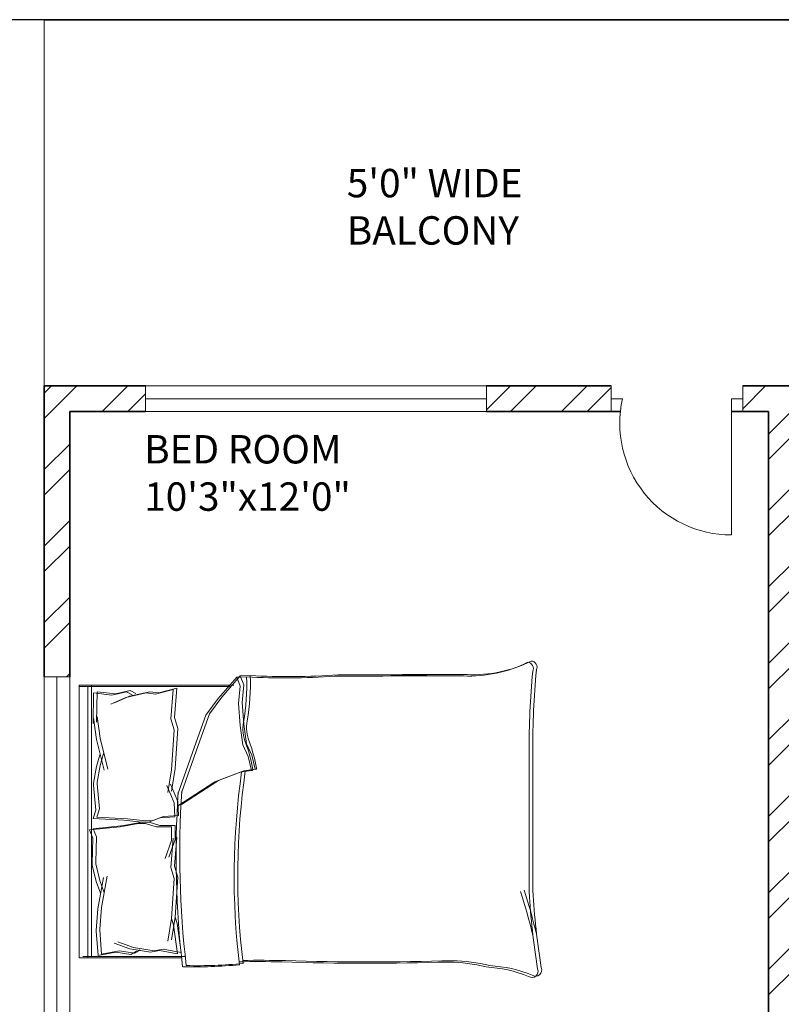
# Model space of a CAD drawing. Units: inches. Extents: x 2168 to 3056, y 1130 to 2629.
# Tile 23 of 42: x 2327 to 2462, y 2305 to 2478. Entities that reach past the tile are written whole.
import ezdxf

# ---------------------------------------------------------------- set-up
doc = ezdxf.new("R2010")
doc.units = ezdxf.units.IN
for name, color, linetype, lineweight in [('A-ANNO-DIMS', 2, 'Continuous', 18), ('A-AREA-IDEN', 7, 'Continuous', 18), ('A-DOOR', 21, 'Continuous', 18), ('A-FLOR-OTLN', 7, 'Continuous', 18), ('A-FURN', 8, 'Continuous', 13), ('A-GLAZ', 201, 'Continuous', 18), ('A-WALL', 7, 'Continuous', 35)]:
    doc.layers.add(name, color=color, linetype=linetype, lineweight=lineweight)
doc.layers.add('A-WALL-PATT', color=143, linetype='Continuous', lineweight=13, true_color=0x7aafdf)
doc.styles.get("Standard").update_dxf_attribs({"font": 'arial.ttf'})
doc.dimstyles.get("Standard").update_dxf_attribs({"dimtxt": 0.18, "dimasz": 0.18, "dimexe": 0.18, "dimexo": 0.0625, "dimgap": 0.09, "dimtad": 0, "dimtih": 1, "dimtoh": 1, "dimdec": 4, "dimzin": 0, "dimdsep": 46, "dimtxsty": 'Standard', "dimcen": 0.09, "dimadec": 0, "dimazin": 0, "dimtfac": 1, "dimtdec": 4, "dimtofl": 0, "dimtmove": 0, "dimatfit": 3, "dimfxl": 1, "dimtolj": 1, "dimtzin": 0, "dimarcsym": 0})

# ---------------------------------------------------------------- blocks, each defined once
blk = doc.blocks.new('BED-DOUBLE')
for p, q in [((27.75, 52.87), (24.5, 49.16)), ((27.75, 52.87), (24.5, 49.16)), ((28.39, 53.1), (25.14, 49.39)), ((28.39, 53.1), (25.14, 49.39)), ((29.49, 52.95), (27.75, 52.87, 3.87)), ((29.49, 52.95), (27.75, 52.87, 3.87)), ((28.37, 51.33), (27.75, 52.87)), ((28.37, 51.33), (27.75, 52.87)), ((30.13, 53.18), (28.39, 53.1, 3.87)), ((30.13, 53.18), (28.39, 53.1, 3.87)), ((29, 51.56), (28.39, 53.1)), ((29, 51.56), (28.39, 53.1)), ((0, 51.49), (0.64, 51.49)), ((0, 3.48), (0, 51.49)), ((0, 51.27), (26.61, 51.27)), ((0, 51.27), (26.61, 51.27)), ((0.64, 51.49), (27.25, 51.49)), ((0.64, 51.49), (27.25, 51.49)), ((1.53, 3.48), (1.53, 51.27)), ((1.53, 3.48), (1.53, 51.27)), ((2.17, 3.7), (2.17, 51.49)), ((2.17, 3.7), (2.17, 51.49)), ((3.2, 50.34), (3.1, 44.94)), ((3.2, 50.34), (3.1, 44.94)), ((3.2, 50.34), (6.41, 49.96)), ((3.2, 50.34), (6.41, 49.96)), ((5.77, 49.73), (8.34, 50.33)), ((5.77, 49.73), (8.34, 50.33)), ((6.41, 49.96), (8.98, 50.56)), ((6.41, 49.96), (8.98, 50.56)), ((8.34, 50.33), (9.38, 49.81)), ((8.34, 50.33), (9.38, 49.81)), ((12.47, 50.34), (8.9, 49.54)), ((12.47, 50.34), (8.9, 49.54)), ((8.98, 50.56), (10.02, 50.04)), ((8.98, 50.56), (10.02, 50.04)), ((14.07, 50.15), (12.47, 50.34)), ((14.07, 50.15), (12.47, 50.34)), ((16.57, 50.7), (13.43, 49.92)), ((16.57, 50.7), (13.43, 49.92)), ((17.21, 50.93), (14.07, 50.15)), ((17.21, 50.93), (14.07, 50.15)), ((16.17, 45.57), (16.57, 50.7)), ((16.17, 45.57), (16.57, 50.7)), ((16.81, 45.8), (17.21, 50.93)), ((16.81, 45.79), (17.21, 50.93)), ((28.06, 48.23), (28.37, 51.33)), ((28.06, 48.23), (28.37, 51.33)), ((28.7, 48.46), (29, 51.56)), ((28.7, 48.46), (29, 51.56)), ((2.56, 50.11), (2.46, 44.71)), ((2.56, 50.11), (2.46, 44.71)), ((2.56, 50.11), (5.77, 49.73)), ((2.56, 50.11), (5.77, 49.73)), ((8.26, 49.31), (5.58, 48.13)), ((8.26, 49.31), (5.58, 48.13)), ((8.9, 49.54), (6.22, 48.36)), ((8.9, 49.54), (6.22, 48.36)), ((11.83, 50.11), (8.26, 49.31)), ((11.83, 50.11), (8.26, 49.31)), ((13.43, 49.92), (11.83, 50.11)), ((13.43, 49.92), (11.83, 50.11)), ((24.5, 49.16), (22.33, 46.22)), ((24.5, 49.16), (22.33, 46.22)), ((25.14, 49.39), (22.97, 46.45)), ((25.14, 49.39), (22.97, 46.45)), ((28.37, 44.36), (28.06, 48.23)), ((28.37, 44.36), (28.06, 48.23)), ((29, 44.59), (28.7, 48.46)), ((29, 44.59), (28.7, 48.46)), ((2.46, 44.71), (2.54, 45.71)), ((2.46, 44.71), (2.54, 45.71)), ((2.54, 45.71), (3.07, 41.91)), ((2.54, 45.71), (3.07, 41.91)), ((3.1, 44.94), (3.18, 45.94)), ((3.1, 44.94), (3.18, 45.94)), ((3.18, 45.94), (3.71, 42.14)), ((3.18, 45.94), (3.71, 42.14)), ((16.73, 43.61), (16.17, 45.57)), ((16.73, 43.61), (16.17, 45.57)), ((17.37, 43.83), (16.81, 45.8)), ((17.37, 43.83), (16.81, 45.79)), ((22.33, 46.22), (20.32, 40.64)), ((22.33, 46.22), (20.32, 40.64)), ((22.97, 46.45), (20.96, 40.87)), ((22.97, 46.45), (20.96, 40.87)), ((16.3, 36.6), (16.73, 43.61)), ((16.3, 36.6), (16.73, 43.61)), ((16.93, 36.82), (17.37, 43.83)), ((16.93, 36.82), (17.37, 43.83)), ((28.83, 40.95), (28.37, 44.36)), ((28.83, 40.95), (28.37, 44.36)), ((29.47, 41.18), (29, 44.59)), ((29.47, 41.18), (29, 44.59)), ((3.07, 41.91), (4.42, 36.5)), ((3.07, 41.91), (4.42, 36.49)), ((3.71, 42.14), (5.06, 36.72)), ((3.71, 42.14), (5.06, 36.72)), ((20.32, 40.64), (17.38, 32.31)), ((20.32, 40.64), (17.38, 32.31)), ((20.96, 40.87), (18.02, 32.53)), ((20.96, 40.87), (18.02, 32.53)), ((29.76, 38.94), (28.83, 40.95)), ((29.76, 38.94), (28.83, 40.95)), ((30.4, 39.17), (29.47, 41.18)), ((30.4, 39.17), (29.47, 41.18)), ((79.88, 15.29), (79.88, 39.91)), ((79.88, 15.29), (79.88, 39.91)), ((3.67, 39.2), (3.08, 37.14)), ((3.67, 39.2), (3.08, 37.14)), ((4.31, 39.43), (3.72, 37.36)), ((4.31, 39.43), (3.72, 37.36)), ((30.38, 36.46), (29.76, 38.94)), ((30.38, 36.46), (29.76, 38.94)), ((31.02, 36.69), (30.4, 39.17)), ((31.02, 36.69), (30.4, 39.17)), ((79.25, 15.06), (79.25, 39.68)), ((79.25, 15.06), (79.25, 39.68)), ((3.08, 37.14), (2.54, 34.2)), ((3.08, 37.14), (2.54, 34.2)), ((3.72, 37.36), (3.18, 34.43)), ((3.72, 37.36), (3.18, 34.43)), ((15.63, 32.56), (16.3, 36.6)), ((15.63, 32.56), (16.3, 36.6)), ((16.27, 32.79), (16.93, 36.82)), ((16.27, 32.79), (16.93, 36.82)), ((28.37, 36.15), (30.38, 36.46)), ((28.37, 36.15), (30.38, 36.46)), ((29, 36.38), (31.02, 36.69)), ((29, 36.38), (31.02, 36.69)), ((23.88, 34.45), (28.37, 36.15)), ((23.88, 34.45), (28.37, 36.15)), ((24.52, 34.68), (29, 36.38)), ((24.52, 34.68), (29, 36.38)), ((2.54, 34.2), (2.56, 33.88)), ((2.54, 34.2), (2.56, 33.88)), ((2.56, 33.88), (2.98, 29.46)), ((2.56, 33.88), (2.98, 29.46)), ((3.18, 34.43), (3.2, 34.11)), ((3.18, 34.43), (3.2, 34.11)), ((3.2, 34.11), (3.62, 29.68)), ((3.2, 34.11), (3.62, 29.68)), ((16.74, 30.75), (15.45, 33.82)), ((16.74, 30.75), (15.45, 33.82)), ((17.38, 30.98), (16.09, 34.05)), ((17.38, 30.98), (16.09, 34.05)), ((17.38, 30.26), (23.88, 34.45)), ((17.38, 30.26), (23.88, 34.45)), ((18.02, 30.49), (24.52, 34.68)), ((18.02, 30.49), (24.52, 34.68)), ((3.62, 29.68), (3.13, 28.21)), ((3.62, 29.68), (3.13, 28.21)), ((16.89, 28.3), (16.74, 30.75)), ((16.89, 28.3), (16.74, 30.75)), ((17.53, 28.53), (17.38, 30.98)), ((17.53, 28.53), (17.38, 30.98)), ((2.98, 29.46), (2.49, 27.98)), ((2.98, 29.46), (2.49, 27.98)), ((2.49, 27.98), (7.87, 27.73)), ((2.49, 27.98), (7.87, 27.73)), ((3.13, 28.21), (8.51, 27.96)), ((3.13, 28.21), (8.51, 27.96)), ((8.51, 27.96), (11.72, 27.58)), ((8.51, 27.96), (11.72, 27.58)), ((12.38, 27.44), (14.22, 28.13)), ((12.38, 27.44), (14.22, 28.13)), ((13.02, 27.66), (14.86, 28.36)), ((13.02, 27.66), (14.86, 28.36)), ((14.22, 28.13), (16.89, 28.3)), ((14.22, 28.13), (16.89, 28.3)), ((14.86, 28.36), (17.53, 28.53)), ((14.86, 28.36), (17.53, 28.53)), ((1.87, 25.98), (7.22, 26.56)), ((1.87, 25.98), (7.22, 26.56)), ((2.51, 26.21), (7.86, 26.79)), ((2.51, 26.21), (7.86, 26.79)), ((3.09, 24.77), (2.51, 26.21)), ((3.09, 24.77), (2.51, 26.21)), ((7.22, 26.56), (10.4, 27.14)), ((7.22, 26.56), (10.4, 27.14)), ((7.86, 26.79), (11.04, 27.37)), ((7.86, 26.79), (11.04, 27.37)), ((7.87, 27.73), (11.08, 27.36)), ((7.87, 27.73), (11.08, 27.35)), ((10.4, 27.14), (11.7, 27.14)), ((10.4, 27.14), (11.7, 27.14)), ((11.04, 27.37), (12.34, 27.37)), ((11.04, 27.37), (12.34, 27.37)), ((11.08, 27.36), (12.38, 27.44)), ((11.08, 27.35), (12.38, 27.44)), ((11.7, 27.14), (13.58, 26.56)), ((11.7, 27.14), (13.58, 26.56)), ((11.72, 27.58), (13.02, 27.66)), ((11.72, 27.58), (13.02, 27.66)), ((12.34, 27.37), (14.22, 26.79)), ((12.34, 27.37), (14.22, 26.79)), ((13.58, 26.56), (16.26, 26.56)), ((13.58, 26.56), (16.26, 26.56)), ((14.22, 26.79), (16.9, 26.79)), ((14.22, 26.79), (16.9, 26.79)), ((16.26, 26.56), (16.26, 24.1)), ((16.26, 26.56), (16.26, 24.1)), ((16.9, 26.79), (16.9, 24.33)), ((16.9, 26.79), (16.9, 24.33)), ((2.45, 24.54), (1.87, 25.98)), ((2.45, 24.54), (1.87, 25.98)), ((2.3, 20.09), (2.45, 24.54)), ((2.3, 20.09), (2.45, 24.54)), ((2.94, 20.32), (3.09, 24.77)), ((2.94, 20.32), (3.09, 24.77)), ((16.9, 24.33), (15.81, 21.19)), ((16.9, 24.33), (15.81, 21.19)), ((16.17, 19.38), (16.57, 24.52)), ((16.17, 19.38), (16.57, 24.52)), ((16.81, 19.61), (17.21, 24.74)), ((16.81, 19.61), (17.21, 24.74)), ((16.26, 24.1), (15.17, 20.96)), ((16.26, 24.1), (15.17, 20.96)), ((2.3, 19.77), (2.3, 20.09)), ((2.3, 19.77), (2.3, 20.09)), ((3.03, 16.88), (2.3, 19.77)), ((3.03, 16.88), (2.3, 19.77)), ((2.94, 20), (2.94, 20.32)), ((2.94, 20), (2.94, 20.32)), ((3.67, 17.11), (2.94, 20)), ((3.67, 17.11), (2.94, 20)), ((16.73, 17.42), (16.17, 19.38)), ((16.73, 17.42), (16.17, 19.38)), ((17.37, 17.65), (16.81, 19.61)), ((17.37, 17.65), (16.81, 19.61)), ((3.32, 12.11), (4.33, 17.6)), ((3.32, 12.11), (4.33, 17.6)), ((3.96, 12.34), (4.97, 17.83)), ((3.96, 12.34), (4.97, 17.83)), ((16.3, 10.41), (16.73, 17.42)), ((16.3, 10.41), (16.73, 17.42)), ((16.93, 10.64), (17.37, 17.65)), ((16.93, 10.64), (17.37, 17.65)), ((3.75, 14.86), (3.03, 16.88)), ((3.75, 14.85), (3.03, 16.88)), ((4.39, 15.08), (3.67, 17.11)), ((4.39, 15.08), (3.67, 17.11)), ((3.67, 8.51), (3.96, 12.34)), ((3.67, 8.51), (3.96, 12.34)), ((3.03, 8.29), (3.32, 12.11)), ((3.03, 8.28), (3.32, 12.11)), ((15.63, 6.38), (16.3, 10.41)), ((15.63, 6.38), (16.3, 10.41)), ((16.27, 6.61), (16.93, 10.64)), ((16.27, 6.61), (16.93, 10.64)), ((16.3, 10.41), (16.62, 9.28)), ((16.3, 10.41), (16.62, 9.28)), ((16.93, 10.64), (17.26, 9.51)), ((16.93, 10.64), (17.26, 9.51)), ((16.62, 9.28), (17.34, 4.18)), ((16.62, 9.28), (17.34, 4.18)), ((17.26, 9.51), (17.98, 4.41)), ((17.26, 9.51), (17.98, 4.41)), ((3.01, 8.18), (3.03, 8.29)), ((3.01, 8.18), (3.03, 8.28)), ((3.34, 3.9), (3.01, 8.18)), ((3.34, 3.9), (3.01, 8.18)), ((3.65, 8.41), (3.67, 8.51)), ((3.65, 8.41), (3.67, 8.51)), ((3.98, 4.13), (3.65, 8.41)), ((3.98, 4.13), (3.65, 8.41)), ((8.96, 5.05), (6.21, 6.06)), ((8.96, 5.05), (6.21, 6.06)), ((9.59, 5.28), (6.85, 6.29)), ((9.59, 5.28), (6.85, 6.29)), ((13.21, 4.7), (9.59, 5.28)), ((13.21, 4.7), (9.59, 5.28)), ((18.11, 3.48), (0, 3.48)), ((18.11, 3.48), (0, 3.48)), ((18.75, 3.7), (0.64, 3.7)), ((18.75, 3.7), (0.64, 3.7)), ((3.32, 3.89), (6.5, 4.47)), ((3.32, 3.89), (6.5, 4.47)), ((3.96, 4.12), (7.14, 4.7)), ((3.96, 4.12), (7.14, 4.7)), ((6.5, 4.47), (9.1, 4.04)), ((6.5, 4.47), (9.1, 4.04)), ((7.14, 4.7), (9.74, 4.27)), ((7.14, 4.7), (9.74, 4.27)), ((12.57, 4.47), (8.96, 5.05)), ((12.57, 4.47), (8.96, 5.05)), ((9.1, 4.04), (10.11, 4.62)), ((9.1, 4.04), (10.11, 4.62)), ((9.74, 4.27), (10.75, 4.85)), ((9.74, 4.27), (10.75, 4.85)), ((14.16, 4.76), (12.57, 4.47)), ((14.16, 4.76), (12.57, 4.47)), ((14.8, 4.99), (13.21, 4.7)), ((14.8, 4.99), (13.21, 4.7)), ((17.34, 4.18), (14.16, 4.76)), ((17.34, 4.18), (14.16, 4.76)), ((17.98, 4.41), (14.8, 4.99)), ((17.98, 4.41), (14.8, 4.99))]:
    blk.add_line(p, q)
for centre, radius, start, end in [((68.67, 76.16), 23.07, 267.4714, 296.4681), ((68.67, 76.16), 23.07, 267.4714, 296.4681), ((69.31, 76.39), 23.07, 267.4714, 296.4681), ((69.31, 76.39), 23.07, 267.4714, 296.4681), ((78.87, 54.41), 1.1, 332.6588, 86.02), ((78.87, 54.41), 1.1, 332.6588, 86.02), ((79.51, 54.64), 1.1, 332.6588, 86.02), ((79.51, 54.64), 1.1, 332.6588, 86.02), ((212.28, 41.15), 133.04, 174.4998, 180.6351), ((212.28, 41.15), 133.04, 174.4998, 180.6351), ((212.92, 41.38), 133.04, 174.4998, 180.6351), ((212.92, 41.38), 133.04, 174.4998, 180.6351), ((-6.66, 51.33), 36.18, 349.8763, 2.5657), ((-6.66, 51.33), 36.18, 349.8763, 2.5657), ((36.32, 182.27), 129.5, 266.9791, 273.8365), ((36.32, 182.27), 129.5, 266.9791, 273.8365), ((-6.02, 51.56), 36.18, 349.8763, 2.5657), ((-6.02, 51.56), 36.18, 349.8763, 2.5657), ((36.95, 182.49), 129.5, 266.9791, 273.8365), ((36.95, 182.49), 129.5, 266.9791, 273.8365), ((67.82, -4508.74), 4561.86, 90.00217, 90.28689), ((67.82, -4508.74), 4561.86, 90.00217, 90.28689), ((68.46, -4508.51), 4561.86, 90.00217, 90.28689), ((68.46, -4508.52), 4561.86, 90.00217, 90.28689), ((35.71, 43.97), 6.22, 168.6608, 203.7384), ((35.71, 43.97), 6.22, 168.6608, 203.7384), ((35.07, 43.74), 6.22, 168.6608, 203.7384), ((35.07, 43.74), 6.22, 168.6608, 203.7384), ((1.48, 31.15), 29.65, 10.6617, 19.8806), ((1.48, 31.15), 29.65, 10.6617, 19.8806), ((2.12, 31.38), 29.65, 10.6617, 19.8806), ((2.12, 31.38), 29.65, 10.6617, 19.8806), ((156.96, 17.98), 129.02, 171.7845, 186.9006), ((156.96, 17.98), 129.02, 171.7845, 186.9006), ((30.44, 36.64), 0.185, 250.2464, 1.1377), ((30.44, 36.64), 0.185, 250.2464, 1.1377), ((31.08, 36.86), 0.185, 250.2464, 1.1377), ((31.08, 36.86), 0.185, 250.2464, 1.1377), ((156.32, 17.76), 129.02, 171.7845, 186.9006), ((156.32, 17.76), 129.02, 171.7845, 186.9006), ((182.05, 21.36), 164.97, 176.0865, 186.7821), ((182.05, 21.36), 164.97, 176.0865, 186.7821), ((182.69, 21.59), 164.97, 176.0865, 186.7821), ((182.69, 21.59), 164.97, 176.0865, 186.7821), ((-23.71, -17.22), 106.46, 13.3832, 17.7053), ((-23.71, -17.22), 106.46, 13.3832, 17.7053), ((-23.07, -16.99), 106.46, 13.3832, 17.7053), ((-23.07, -16.99), 106.46, 13.3832, 17.7053), ((200.84, 21.43), 121.76, 182.9958, 189.4091), ((200.84, 21.43), 121.76, 182.9958, 189.4091), ((201.48, 21.66), 121.76, 182.9958, 189.4091), ((201.48, 21.66), 121.76, 182.9958, 189.4091), ((20.1, 85.16), 83.31, 268.7218, 275.604), ((20.1, 85.16), 83.31, 268.7218, 275.604), ((20.74, 85.39), 83.31, 268.7218, 275.604), ((20.74, 85.39), 83.31, 268.7218, 275.604), ((31.17, -167.31), 170.11, 88.4762, 91.0082), ((31.17, -167.31), 170.11, 88.4762, 91.0082), ((31.81, -167.08), 170.11, 88.4762, 91.0082), ((31.81, -167.08), 170.11, 88.4762, 91.0082), ((50.61, 484.82), 482.31, 268.2277, 271.7185), ((50.61, 484.82), 482.31, 268.2277, 271.7185), ((51.25, 485.05), 482.31, 268.2277, 271.7185), ((51.25, 485.05), 482.31, 268.2277, 271.7185), ((64.52, -26.9), 29.63, 76.0648, 88.9113), ((64.52, -26.9), 29.63, 76.0648, 88.9113), ((65.15, -26.67), 29.63, 76.0648, 88.9113), ((65.15, -26.67), 29.63, 76.0648, 88.9113), ((70.28, -21.66), 23.56, 67.9751, 86.652), ((70.28, -21.66), 23.56, 67.9751, 86.652), ((70.92, -21.43), 23.56, 67.9751, 86.652), ((70.92, -21.43), 23.56, 67.9751, 86.652), ((80.36, 1.32), 1.09, 236.1736, 23.4781), ((80.36, 1.32), 1.09, 236.1736, 23.4781), ((79.72, 1.09), 1.09, 236.1736, 23.4781), ((79.72, 1.09), 1.09, 236.1736, 23.4781)]:
    blk.add_arc(centre, radius, start, end)
blk = doc.blocks.new('WIN-60-OPPOSED-JAMBS')
for p, q in [((2.25, 60), (0, 60)), ((0, 60), (4.5, 60)), ((0, 60), (0, 0)), ((2.25, 0), (2.25, 60)), ((4.5, 60), (4.5, 0)), ((0, 0), (4.5, 0)), ((4.5, 0), (2.25, 0))]:
    blk.add_line(p, q)
blk = doc.blocks.new('*D41')
at = {"layer": 'A-ANNO-DIMS', "color": 0, "lineweight": -2, "transparency": 16777216}
for p, q in [((2331.73, 2478.39), (2273.32, 2478.39)), ((2273.5, 2478.21), (2273.5, 1928.07)), ((2273.5, 1377.57), (2273.5, 1927.71)), ((2331.73, 1377.39), (2273.32, 1377.39))]:
    blk.add_line(p, q, dxfattribs=at)
at = {"layer": 'A-ANNO-DIMS', "color": 0, "transparency": 16777216}
for points in [[(2273.47, 2478.21), (2273.53, 2478.21), (2273.5, 2478.39)], [(2273.47, 1377.57), (2273.53, 1377.57), (2273.5, 1377.39)]]:
    blk.add_solid(points, dxfattribs=at)
at = {"layer": 'Defpoints', "color": 0, "transparency": 16777216}
for p in [(2273.5, 2478.39), (2331.8, 2478.39), (2331.8, 1377.39)]:
    blk.add_point(p, dxfattribs=at)
at = {"layer": 'A-ANNO-DIMS', "color": 0, "transparency": 16777216, "insert": (2273.5, 1927.89), "char_height": 0.18, "attachment_point": 5}
blk.add_mtext('\\A1;1101', dxfattribs=at)

msp = doc.modelspace()

# ---------------------------------------------------------------- hatches: boundary and pattern name
at = {"layer": 'A-WALL-PATT'}
h = msp.add_hatch(dxfattribs=at)
h.set_pattern_fill('ANSI32', color=256)
h.paths.add_polyline_path([(2463.8, 2409.39), (2467.39, 2409.39), (2467.39, 2413.89), (2454.77, 2413.89), (2454.77, 2411.64), (2454.77, 2409.39), (2459.3, 2409.39), (2459.3, 2265.39), (2455.64, 2265.39), (2455.64, 2260.89), (2467.35, 2260.89), (2467.35, 2263.14), (2467.35, 2265.39), (2463.8, 2265.39)])
h.paths.add_polyline_path([(2431.6, 2413.89), (2409.65, 2413.89), (2409.65, 2409.39), (2431.6, 2409.39), (2431.6, 2411.64)])
h.paths.add_polyline_path([(2349.65, 2413.89), (2331.8, 2413.89), (2331.8, 2362.67), (2336.3, 2362.67), (2336.3, 2409.39), (2349.65, 2409.39), (2349.65, 2411.64)])
h.paths.add_polyline_path([(2634.15, 2411.64), (2634.15, 2413.89), (2562.29, 2413.89), (2562.29, 2409.39), (2595.8, 2409.39), (2595.8, 2280.31), (2595.83, 2280.31), (2595.83, 2265.39), (2499.91, 2265.39), (2499.91, 2260.89), (2550.8, 2260.89), (2550.8, 2117.31), (2555.3, 2117.31), (2555.3, 2168.08), (2571.93, 2168.08), (2571.93, 2176.89), (2559.8, 2176.89), (2559.8, 2256.39), (2640.8, 2256.39), (2640.8, 2176.89), (2626.43, 2176.89), (2626.43, 2168.08), (2645.3, 2168.08), (2645.3, 2116.64), (2649.8, 2116.64), (2649.8, 2260.89), (2691.25, 2260.89), (2691.25, 2263.14), (2691.25, 2265.39), (2670.65, 2265.39), (2670.65, 2265.36), (2600.3, 2265.36), (2600.3, 2280.26), (2600.3, 2409.39), (2634.15, 2409.39)])
h.paths.add_polyline_path([(2600.3, 2473.89), (2612.84, 2473.89), (2612.84, 2478.39), (2572.64, 2478.39), (2572.64, 2473.89), (2595.8, 2473.89), (2595.8, 2413.89), (2600.3, 2413.89)])
h.paths.add_polyline_path([(2535.8, 2473.89), (2548.64, 2473.89), (2548.64, 2478.39), (2531.4, 2478.39), (2531.4, 2413.89), (2521.6, 2413.89), (2521.6, 2409.39), (2539.24, 2409.39), (2539.24, 2411.64), (2539.24, 2413.89), (2535.8, 2413.89)])
h.paths.add_polyline_path([(2664.8, 2478.39), (2636.84, 2478.39), (2636.84, 2473.89), (2660.3, 2473.89), (2660.3, 2413.89), (2656.17, 2413.89), (2656.17, 2409.39), (2671.68, 2409.39), (2671.68, 2411.64), (2671.68, 2413.89), (2664.8, 2413.89)])
h.paths.add_polyline_path([(2705.94, 2413.89), (2695.68, 2413.89), (2695.68, 2409.39), (2705.94, 2409.39)])
h.paths.add_polyline_path([(2741.35, 2413.89), (2728.73, 2413.89), (2728.73, 2411.64), (2728.73, 2409.39), (2732.3, 2409.39), (2732.3, 2265.39), (2725.73, 2265.39), (2725.73, 2260.89), (2740.92, 2260.89), (2740.92, 2263.14), (2740.92, 2265.39), (2736.8, 2265.39), (2736.8, 2409.39), (2741.35, 2409.39)])
h.paths.add_polyline_path([(2785.65, 2413.89), (2764.55, 2413.89), (2764.49, 2409.39), (2785.65, 2409.39), (2785.65, 2411.64)])
h.paths.add_polyline_path([(2864.3, 2413.89), (2845.65, 2413.89), (2845.65, 2409.39), (2859.8, 2409.39), (2859.8, 2368.43), (2864.3, 2368.43)])
h.paths.add_polyline_path([(2864.3, 2308.43), (2862.05, 2308.43), (2859.8, 2308.43), (2859.8, 2265.39), (2774.48, 2265.39), (2774.48, 2263.14), (2774.48, 2260.89), (2781.8, 2260.89), (2781.8, 2226.65), (2786.3, 2226.65), (2786.3, 2260.89), (2859.8, 2260.89), (2859.8, 2241.35), (2864.3, 2241.35)])
h.paths.add_polyline_path([(2864.3, 2217.35), (2862.05, 2217.35), (2859.8, 2217.35), (2859.8, 2200.89), (2786.3, 2200.89), (2786.3, 2205.93), (2784.05, 2205.93), (2781.8, 2205.93), (2781.8, 2150.97), (2786.3, 2150.97), (2786.3, 2161.89), (2859.8, 2161.89), (2859.8, 2144.42), (2864.3, 2144.42)])
h.paths.add_polyline_path([(2859.8, 2196.39), (2859.8, 2166.39), (2786.3, 2166.39), (2786.3, 2196.39)], flags=16)
h.paths.add_polyline_path([(2864.3, 2108.42), (2862.05, 2108.42), (2859.8, 2108.42), (2859.8, 2080.89), (2786.3, 2080.89), (2786.3, 2111.99), (2781.8, 2111.99), (2781.8, 2080.89), (2649.8, 2080.89), (2649.8, 2086.04), (2647.55, 2086.04), (2645.3, 2086.04), (2645.3, 2071.74), (2649.8, 2071.74), (2649.8, 2076.39), (2781.8, 2076.39), (2781.8, 2041.79), (2786.3, 2041.79), (2786.3, 2076.39), (2859.8, 2076.39), (2859.8, 2058.58), (2864.3, 2058.58)])
h.paths.add_polyline_path([(2864.3, 2022.58), (2859.8, 2022.58), (2859.8, 1992.39), (2786.3, 1992.39), (2786.3, 1999.57), (2781.8, 1999.57), (2781.8, 1848.09), (2784.05, 1848.09), (2786.3, 1848.09), (2786.3, 1851.39), (2859.8, 1851.39), (2859.8, 1838.26), (2864.3, 1838.26)], flags=17)
h.paths.add_polyline_path([(2859.8, 1987.89), (2859.8, 1855.89), (2786.3, 1855.89), (2786.3, 1987.89)], flags=16)
h.paths.add_polyline_path([(2823.05, 1987.89), (2841.42, 1921.89), (2823.05, 1855.89)], flags=0)
h.paths.add_polyline_path([(2864.3, 1814.26), (2859.8, 1814.26), (2859.8, 1791.39), (2786.3, 1791.39), (2786.3, 1825.66), (2784.05, 1825.66), (2781.8, 1825.66), (2781.8, 1791.39), (2720.15, 1791.39), (2720.15, 1791.27), (2649.8, 1791.27), (2649.8, 1806.16), (2649.8, 2038.98), (2647.55, 2038.98), (2645.3, 2038.98), (2645.3, 1783.93), (2649.8, 1783.93), (2649.8, 1786.89), (2781.8, 1786.89), (2781.8, 1746.79), (2786.3, 1746.79), (2786.3, 1786.89), (2859.8, 1786.89), (2859.8, 1770.08), (2864.3, 1770.08)])
h.paths.add_polyline_path([(2864.3, 1734.08), (2862.05, 1734.08), (2859.8, 1734.08), (2859.8, 1705.89), (2786.3, 1705.89), (2786.3, 1714.17), (2781.8, 1714.17), (2781.8, 1660.53), (2786.3, 1660.53), (2786.3, 1666.89), (2859.8, 1666.89), (2859.8, 1648.34), (2864.3, 1648.34)])
h.paths.add_polyline_path([(2786.3, 1701.39), (2859.8, 1701.39), (2859.8, 1671.39), (2786.3, 1671.39)], flags=16)
h.paths.add_polyline_path([(2649.8, 1756.58), (2647.55, 1756.58), (2645.3, 1756.58), (2645.3, 1606.89), (2555.3, 1606.89), (2555.3, 1749.51), (2553.05, 1749.51), (2550.8, 1749.51), (2550.8, 1606.89), (2503.01, 1606.89), (2503.01, 1604.64), (2503.01, 1602.39), (2595.8, 1602.39), (2595.85, 1602.39), (2595.85, 1587.5), (2595.8, 1458.39), (2561.5, 1458.39), (2561.5, 1456.14), (2561.5, 1453.89), (2595.8, 1453.89), (2595.8, 1381.89), (2573.44, 1381.89), (2573.44, 1377.39), (2613.01, 1377.39), (2613.01, 1379.64), (2613.01, 1381.89), (2600.3, 1381.89), (2600.3, 1453.89), (2634.33, 1453.89), (2634.33, 1458.39), (2600.3, 1458.39), (2600.3, 1602.39), (2670.65, 1602.39), (2694.09, 1602.39), (2694.09, 1606.89), (2649.8, 1606.89)])
h.paths.add_polyline_path([(2736.8, 1602.39), (2741.56, 1602.39), (2741.56, 1606.89), (2726.2, 1606.89), (2726.2, 1604.64), (2726.2, 1602.39), (2732.3, 1602.39), (2732.3, 1458.39), (2727.9, 1458.39), (2727.9, 1453.89), (2740.82, 1453.89), (2740.82, 1456.14), (2740.82, 1458.39), (2736.8, 1458.39)])
h.paths.add_polyline_path([(2859.8, 1606.89), (2786.3, 1606.89), (2786.3, 1637.33), (2784.05, 1637.33), (2781.8, 1637.33), (2781.8, 1606.89), (2775.61, 1606.89), (2775.61, 1602.39), (2859.8, 1602.39)])
h.paths.add_polyline_path([(2864.3, 1624.34), (2862.05, 1624.34), (2859.8, 1624.34), (2859.8, 1570.39), (2864.3, 1570.39)])
h.paths.add_polyline_path([(2864.3, 1510.39), (2862.05, 1510.39), (2859.8, 1510.39), (2859.8, 1458.39), (2846.73, 1458.39), (2846.73, 1456.14), (2846.73, 1453.89), (2864.3, 1453.89)])
h.paths.add_polyline_path([(2786.73, 1458.39), (2765.44, 1458.39), (2765.44, 1453.89), (2786.73, 1453.89)])
h.paths.add_polyline_path([(2706, 1458.39), (2695.36, 1458.39), (2695.36, 1453.89), (2706, 1453.89), (2706, 1456.14)])
h.paths.add_polyline_path([(2671.36, 1456.14), (2671.36, 1458.39), (2655.99, 1458.39), (2655.99, 1456.14), (2655.99, 1453.89), (2660.3, 1453.89), (2660.3, 1381.89), (2637.01, 1381.89), (2637.01, 1377.39), (2664.8, 1377.39), (2664.8, 1453.89), (2671.36, 1453.89)], flags=17)
h.paths.add_polyline_path([(2539.83, 1458.39), (2520.24, 1458.39), (2520.24, 1453.89), (2531.3, 1453.89), (2531.3, 1377.39), (2546.45, 1377.39), (2546.45, 1379.64), (2546.45, 1381.89), (2535.8, 1381.89), (2535.8, 1453.89), (2539.83, 1453.89)], flags=17)
h.paths.add_polyline_path([(2496.24, 1458.39), (2489.13, 1458.39), (2489.13, 1453.89), (2496.24, 1453.89), (2496.24, 1456.14)])
h.paths.add_polyline_path([(2467.43, 1456.14), (2467.43, 1458.39), (2463.8, 1458.39), (2463.8, 1602.39), (2468.24, 1602.39), (2468.24, 1605.7), (2468.24, 1606.89), (2454.6, 1606.89), (2454.6, 1602.39), (2459.3, 1602.39), (2459.3, 1458.39), (2454.24, 1458.39), (2454.24, 1453.89), (2467.43, 1453.89)])
h.paths.add_polyline_path([(2431.6, 1456.14), (2431.6, 1458.39), (2411.39, 1458.39), (2411.39, 1453.89), (2431.6, 1453.89)])
h.paths.add_polyline_path([(2351.39, 1458.39), (2336.3, 1458.39), (2336.3, 1490.69), (2334.05, 1490.69), (2331.8, 1490.69), (2331.8, 1453.89), (2351.39, 1453.89), (2351.39, 1456.14)])
h.paths.add_polyline_path([(2336.3, 1629.7), (2331.8, 1629.7), (2331.8, 1552.32), (2336.3, 1552.32), (2336.3, 1602.39), (2406.65, 1602.39), (2423.47, 1602.39), (2423.47, 1606.89), (2418.8, 1606.89), (2418.8, 1643.68), (2416.55, 1643.68), (2414.3, 1643.68), (2414.3, 1606.89), (2336.3, 1606.89)])
h.paths.add_polyline_path([(2418.8, 1714.38), (2414.3, 1714.38), (2414.3, 1705.89), (2336.3, 1705.89), (2336.3, 1731.32), (2334.05, 1731.32), (2331.8, 1731.32), (2331.8, 1653.7), (2334.05, 1653.7), (2336.3, 1653.7), (2336.3, 1666.89), (2414.3, 1666.89), (2414.3, 1663.59), (2418.8, 1663.59)])
h.paths.add_polyline_path([(2336.3, 1701.39), (2414.3, 1701.39), (2414.3, 1671.39), (2336.3, 1671.39)], flags=16)
h.paths.add_polyline_path([(2555.3, 2040.06), (2550.8, 2040.06), (2550.8, 1791.39), (2550.56, 1791.2), (2480.2, 1791.2), (2418.8, 1791.39), (2418.8, 1825.45), (2416.55, 1825.45), (2414.3, 1825.45), (2414.3, 1791.39), (2336.3, 1791.39), (2336.3, 1806.41), (2331.8, 1806.41), (2331.8, 1767.32), (2336.3, 1767.32), (2336.3, 1786.89), (2414.3, 1786.89), (2414.3, 1745.46), (2418.8, 1745.46), (2418.8, 1786.89), (2550.8, 1786.89), (2550.8, 1783.01), (2555.3, 1783.01)])
h.paths.add_polyline_path([(2418.8, 1923.39), (2423.21, 1923.39), (2423.21, 1925.64), (2423.21, 1927.89), (2418.8, 1927.89), (2418.8, 2000.05), (2414.3, 2000.05), (2414.3, 1992.39), (2336.3, 1992.39), (2336.3, 1987.89), (2414.3, 1987.89), (2414.3, 1855.89), (2336.3, 1855.89), (2336.3, 1851.39), (2414.3, 1851.39), (2414.3, 1846.76), (2418.8, 1846.76)], flags=17)
h.paths.add_polyline_path([(2336.3, 2019.29), (2334.05, 2019.29), (2331.8, 2019.29), (2331.8, 1830.41), (2336.3, 1830.41)], flags=17)
h.paths.add_polyline_path([(2550.8, 1927.89), (2453.54, 1927.89), (2453.54, 1925.64), (2453.54, 1923.39), (2550.8, 1923.39)], flags=17)
h.paths.add_polyline_path([(2744.99, 1927.89), (2649.8, 1927.89), (2649.8, 1923.39), (2744.99, 1923.39), (2744.99, 1925.64)], flags=17)
h.paths.add_polyline_path([(2555.3, 2086.46), (2553.05, 2086.46), (2550.8, 2086.46), (2550.8, 2080.89), (2418.8, 2080.89), (2336.3, 2080.89), (2336.3, 2115.4), (2334.05, 2115.4), (2331.8, 2115.4), (2331.8, 2055.29), (2336.3, 2055.29), (2336.3, 2076.39), (2550.8, 2076.39), (2550.8, 2071.54), (2555.3, 2071.54)])
h.paths.add_polyline_path([(2418.8, 2121.39), (2414.3, 2121.39), (2414.3, 2080.89), (2418.8, 2080.89)])
h.paths.add_polyline_path([(2418.8, 2076.39), (2414.3, 2076.39), (2414.3, 2035.12), (2418.8, 2035.12)])
h.paths.add_polyline_path([(2422.87, 2263.14), (2422.87, 2265.39), (2406.65, 2265.39), (2406.65, 2265.36), (2336.3, 2265.36), (2336.3, 2280.25), (2336.3, 2302.67), (2334.05, 2302.67), (2331.8, 2302.67), (2331.8, 2246.85), (2336.3, 2246.85), (2336.3, 2260.89), (2414.3, 2260.89), (2414.3, 2224), (2418.8, 2224), (2418.8, 2260.89), (2422.87, 2260.89)])
h.paths.add_polyline_path([(2418.8, 2204.78), (2416.55, 2204.78), (2414.3, 2204.78), (2414.3, 2200.89), (2336.3, 2200.89), (2336.3, 2220.85), (2331.8, 2220.85), (2331.8, 2151.4), (2336.3, 2151.4), (2336.3, 2161.89), (2414.3, 2161.89), (2414.3, 2153.73), (2418.8, 2153.73)])
h.paths.add_polyline_path([(2414.3, 2196.39), (2414.3, 2166.39), (2336.3, 2166.39), (2336.3, 2196.39)], flags=16)
h.paths.add_polyline_path([(2375.3, 2181.39), (2336.3, 2166.39), (2336.3, 2196.39)], flags=0)
h.paths.add_polyline_path([(2809.6, 2172.34), (2838.8, 2172.34), (2838.8, 2191), (2809.6, 2191)], flags=8)
h.paths.add_polyline_path([(2849.75, 1919.59), (2849.75, 1952.67), (2831.09, 1952.67), (2831.09, 1919.59)], flags=8)
h.paths.add_polyline_path([(2808.87, 1901.97), (2808.87, 1937.85), (2790.15, 1937.85), (2790.15, 1901.97)], flags=8)
h.paths.add_polyline_path([(2806.28, 1671.9), (2835.49, 1671.9), (2835.49, 1690.55), (2806.28, 1690.55)], flags=8)
h.paths.add_polyline_path([(2353.19, 1676.55), (2382.39, 1676.55), (2382.39, 1695.21), (2353.19, 1695.21)], flags=8)
h.paths.add_polyline_path([(2360.08, 1832.31), (2389.24, 1832.31), (2389.24, 1850.97), (2360.08, 1850.97)], flags=25)
h.paths.add_polyline_path([(2354.82, 2167.82), (2384.03, 2167.82), (2384.03, 2186.48), (2354.82, 2186.48)], flags=8)

# ---------------------------------------------------------------- linework, layer by layer
at = {"layer": 'A-DOOR'}
for p, q in [((2431.6, 2413.89), (2431.6, 2409.39)), ((2454.77, 2409.39), (2454.77, 2413.89)), ((2454.77, 2413.89), (2454.77, 2413.89)), ((2454.77, 2413.89), (2454.77, 2411.64)), ((2431.6, 2409.39), (2431.6, 2411.64)), ((2431.6, 2411.64), (2433.6, 2411.64)), ((2454.77, 2411.64), (2452.77, 2411.64)), ((2452.77, 2411.64), (2452.77, 2387.64)), ((2454.77, 2409.39), (2454.77, 2409.39))]:
    msp.add_line(p, q, dxfattribs=at)
msp.add_arc((2452.77, 2407.3), 19.66, 167.2377, 270, dxfattribs=at)
at = {"layer": 'A-FLOR-OTLN'}
msp.add_line((2331.8, 2478.39), (2331.8, 2413.89), dxfattribs=at)
at = {"layer": 'A-GLAZ'}
for p, q in [((2349.65, 2409.39), (2349.65, 2413.89)), ((2349.65, 2413.89), (2349.65, 2409.39)), ((2349.65, 2413.89), (2349.65, 2413.89)), ((2349.65, 2413.89), (2409.65, 2413.89)), ((2409.65, 2411.64), (2409.65, 2413.89)), ((2409.65, 2413.89), (2409.65, 2409.39)), ((2349.65, 2409.39), (2349.65, 2411.64)), ((2349.65, 2411.64), (2409.65, 2411.64)), ((2409.65, 2409.39), (2349.65, 2409.39))]:
    msp.add_line(p, q, dxfattribs=at)
at = {"layer": 'A-WALL'}
for p, q in [((2331.8, 2478.39), (2548.64, 2478.39)), ((2331.8, 2413.89), (2349.65, 2413.89)), ((2331.8, 2413.89), (2331.8, 2362.67)), ((2409.65, 2413.89), (2431.6, 2413.89)), ((2454.77, 2413.89), (2467.39, 2413.89)), ((2336.3, 2409.39), (2349.65, 2409.39)), ((2336.3, 2409.39), (2336.3, 2362.67)), ((2409.65, 2409.39), (2433.22, 2409.39)), ((2452.77, 2409.39), (2459.3, 2409.39)), ((2459.3, 2409.39), (2459.3, 2265.39))]:
    msp.add_line(p, q, dxfattribs=at)

# ---------------------------------------------------------------- block references
at = {"layer": 'A-FURN'}
msp.add_blockref('BED-DOUBLE', (2337.94, 2309.7), dxfattribs=at)
at = {"layer": 'A-GLAZ'}
msp.add_blockref('WIN-60-OPPOSED-JAMBS', (2331.8, 2302.67), dxfattribs=at)

# ---------------------------------------------------------------- texts
at = {"layer": 'A-AREA-IDEN', "char_height": 5, "attachment_point": 1}
for s, width, insert in [('5\'0" WIDE\\PBALCONY', 195.8291, (2385.07, 2452.11)), ('BED ROOM\\P10\'3"x12\'0"', 285.8516, (2349.41, 2405.23))]:
    msp.add_mtext_dynamic_manual_height_columns(s, width=width, gutter_width=12.5, heights=[0], dxfattribs=dict(at, insert=insert))

# ---------------------------------------------------------------- dimensions: what is measured, and where the dimension line sits
at = {"layer": 'A-ANNO-DIMS'}
dim = msp.add_linear_dim(base=(2273.5, 2478.39), p1=(2331.8, 1377.39), p2=(2331.8, 2478.39), angle=90, dimstyle='Standard', override={"dimdec": 0, "dimlfac": 1, "dimrnd": 0, "dimzin": 0, "dimdsep": 46, "dimlunit": 2}, dxfattribs=at)
dim.commit()
dim.dimension.update_dxf_attribs({"geometry": '*D41', "text_midpoint": (2273.5, 1927.89)})

doc.saveas('drawing.dxf')
